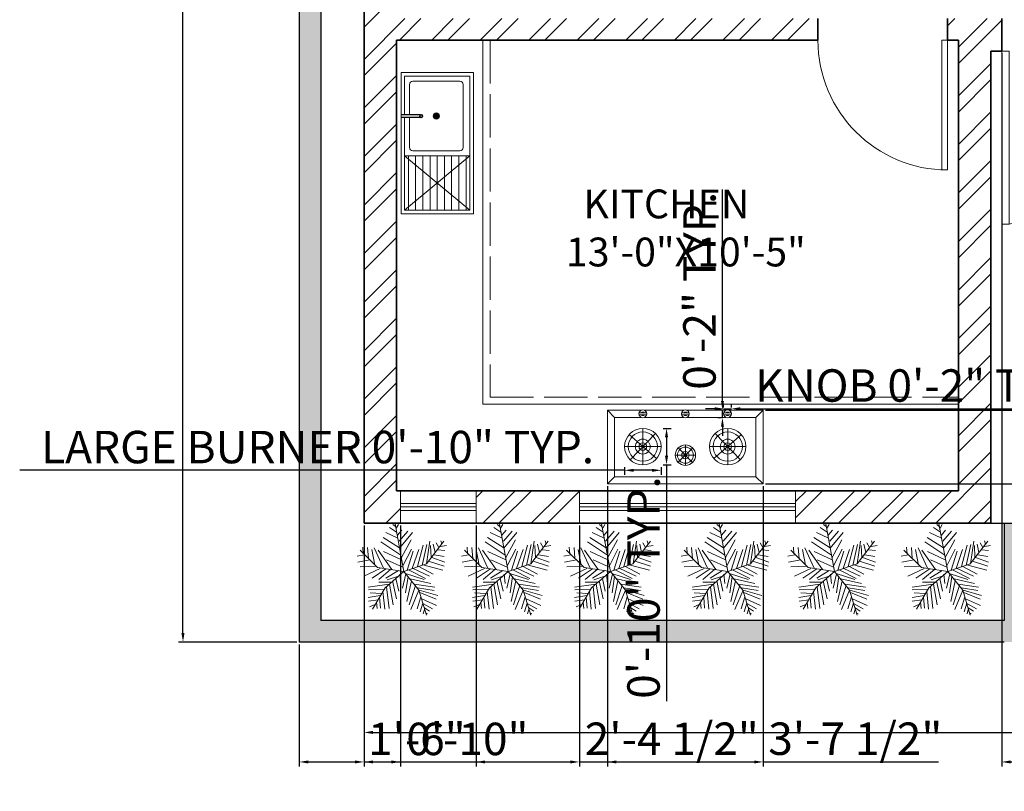
# Model space of a CAD drawing. Units: inches. Extents: x 418 to 1041, y 2094 to 2761.
# Tile 1 of 5: x 450 to 723, y 2094 to 2308. Entities that reach past the tile are written whole.
import ezdxf

# ---------------------------------------------------------------- set-up
doc = ezdxf.new("R2010")
doc.units = ezdxf.units.IN
doc.linetypes.add('ACAD_ISO02W100', pattern=[15, 12, -3])
for name, color, linetype, lineweight in [('A-ANNO-DIMS', 2, 'Continuous', 18), ('A-AREA-IDEN', 7, 'Continuous', 18), ('A-DOOR', 4, 'Continuous', 18), ('A-EQPM', 8, 'Continuous', 18), ('A-FLOR', 7, 'Continuous', 25), ('A-FLOR-CASE', 9, 'Continuous', 18), ('A-FLOR-CASE-HIDN', 9, 'ACAD_ISO02W100', 13), ('A-FLOR-FIXT', 9, 'Continuous', 18), ('A-GLAZ', 244, 'Continuous', 18), ('A-WALL', 7, 'Continuous', 35), ('A-WALL-PATT', 252, 'Continuous', 13), ('L-PLNT', 3, 'Continuous', 13), ('L-WALL', 7, 'Continuous', 25), ('L-WALL-PATT', 252, 'Continuous', 13)]:
    doc.layers.add(name, color=color, linetype=linetype, lineweight=lineweight)
doc.styles.get("Standard").update_dxf_attribs({"font": 'arial.ttf'})
doc.dimstyles.new('ISO-25', dxfattribs={"dimtxt": 9, "dimasz": 2.5, "dimexe": 1.25, "dimexo": 0.625, "dimtad": 1, "dimlunit": 3, "dimtxsty": 'Standard', "dimcen": 2.5, "dimadec": 0, "dimazin": 0, "dimtfac": 1, "dimtmove": 0, "dimatfit": 3, "dimfxl": 1, "dimarcsym": 0})

# ---------------------------------------------------------------- blocks, each defined once
blk = doc.blocks.new('*U3')
for p, q in [((0, 0), (0, 6)), ((40, 0), (40, 6))]:
    blk.add_line(p, q)
blk.add_lwpolyline([(0, 0), (0, -40), (1.75, -40), (1.75, 0)], close=True)
blk.add_arc((0, 0), 40, 270, 0)
blk = doc.blocks.new('*U4')
for p, q in [((-40, 0), (-40, 6)), ((0, 0), (0, 6))]:
    blk.add_line(p, q)
blk.add_lwpolyline([(0, 0), (0, -40), (-1.75, -40), (-1.75, 0)], close=True)
blk.add_arc((0, 0), 40, 180, 270)
blk = doc.blocks.new('*U14')
for p, q in [((-8.737, 47.138), (-17.069, 52.711)), ((-10.186, 53.64), (-13.084, 55.962)), ((0, 0), (-10.5, 57)), ((-9.099, 51.782), (-6.563, 55.962)), ((-7.65, 43.423), (-2.578, 49.46)), ((-5.839, 35.992), (4.667, 48.067)), ((-3.665, 19.273), (-27.574, 35.527)), ((-5.114, 28.097), (-24.676, 40.636)), ((-7.288, 39.707), (-21.778, 46.673)), ((-5.114, 27.632), (10.463, 46.673)), ((-2.941, 16.486), (8.652, 37.85)), ((27, 9), (48, 36)), ((27.127, 9.056), (31.112, 35.992)), ((44.153, 36.456), (45.239, 32.741)), ((-31.5, 4.5), (-52.5, 25.5)), ((-48.585, 21.131), (-49.309, 29.026)), ((-43.513, 28.561), (-42.427, 15.558)), ((-38.442, 26.239), (-34.819, 7.663)), ((-35.544, 28.097), (-24.314, 3.947)), ((-14.533, 2.09), (-30.834, 25.31)), ((-24.314, 23.917), (-2.941, 13.7)), ((-1.129, 6.734), (9.014, 26.704)), ((3.942, 1.625), (11.187, 24.381)), ((10.101, 3.483), (17.708, 26.239)), ((16.259, 5.805), (23.142, 31.348)), ((22.055, 7.198), (27.489, 32.277)), ((31.836, 30.883), (32.561, 16.486)), ((35.096, 32.741), (37.27, 22.524)), ((38.719, 34.134), (41.979, 28.561)), ((40.53, 25.775), (48.862, 24.846)), ((43.791, 29.954), (51.036, 30.883)), ((-47.498, 19.737), (-55.83, 18.344)), ((-40.615, 13.7), (-55.105, 10.913)), ((-20.691, 13.7), (-1.129, 4.876)), ((29.662, 12.307), (48.137, 6.269)), ((33.285, 16.486), (48.862, 10.913)), ((36.183, 19.737), (48.137, 17.88)), ((-33.37, 6.269), (-52.207, 5.34)), ((-28.299, 3.483), (-47.86, -5.805)), ((-21.416, 3.018), (-38.079, -8.128)), ((0, 0), (-31.5, 4.5)), ((-15.982, 2.09), (-30.11, -9.521)), ((0, 0), (-22.5, -19.5)), ((-6.563, 1.161), (-21.416, -8.128)), ((0, 0), (27, 9)), ((0, 0), (18, -22.5)), ((6.478, 1.625), (26.04, -8.592)), ((11.187, 3.483), (30.749, -5.805)), ((18.07, 5.805), (35.096, -3.483)), ((24.229, 7.663), (46.688, 1.625)), ((-6.563, -5.805), (-19.967, -9.985)), ((-13.446, -11.378), (-8.737, -32.741)), ((-9.461, -8.592), (-6.201, -23.453)), ((-4.752, -3.483), (-3.665, -14.629)), ((2.493, -3.019), (-1.491, -20.202)), ((1.769, -2.555), (24.229, -9.521)), ((5.029, -6.27), (2.131, -25.775)), ((9.014, -11.378), (3.58, -35.992)), ((7.565, -9.056), (32.198, -14.629)), ((-17.431, -15.094), (-42.789, -18.809)), ((-24.314, -21.596), (-42.427, -22.06)), ((-22.5, -19.5), (-37.5, -45)), ((-15.257, -12.772), (-30.11, -12.772)), ((-20.691, -18.345), (-17.793, -44.352)), ((-17.069, -15.094), (-12.721, -40.172)), ((14.085, -16.951), (6.478, -40.172)), ((18.07, -22.524), (8.289, -45.745)), ((12.274, -15.094), (36.907, -18.809)), ((16.259, -19.738), (36.183, -22.989)), ((18, -22.5), (27, -52.5)), ((18.433, -22.524), (40.53, -29.026)), ((-28.299, -29.026), (-42.789, -31.348)), ((-30.834, -34.135), (-42.427, -35.528)), ((-26.849, -26.24), (-40.253, -25.775)), ((-29.023, -30.884), (-27.936, -43.887)), ((-25.038, -23.918), (-22.865, -45.281)), ((20.244, -30.419), (15.897, -44.816)), ((19.157, -25.311), (38.719, -33.206)), ((21.331, -32.741), (39.081, -40.636)), ((-34.457, -39.708), (-40.978, -42.494)), ((-32.646, -36.921), (-31.921, -44.352)), ((22.78, -37.85), (19.519, -48.532)), ((22.78, -38.314), (34.372, -44.816)), ((24.591, -45.745), (23.142, -50.854)), ((24.591, -43.423), (30.749, -47.603)), ((26.764, -49.925), (28.213, -50.854))]:
    blk.add_line(p, q)
blk = doc.blocks.new('*D17')
at = {"layer": 'A-ANNO-DIMS', "color": 0, "lineweight": -2, "transparency": 16777216}
for p, q in [((545.56, 2167.4), (545.56, 2108.72)), ((971.56, 2167.4), (971.56, 2108.72)), ((548.06, 2109.97), (969.06, 2109.97))]:
    blk.add_line(p, q, dxfattribs=at)
at = {"layer": 'A-ANNO-DIMS', "color": 0, "transparency": 16777216}
for points in [[(548.06, 2110.39), (548.06, 2109.55), (545.56, 2109.97)], [(969.06, 2110.39), (969.06, 2109.55), (971.56, 2109.97)]]:
    blk.add_solid(points, dxfattribs=at)
at = {"layer": 'Defpoints', "color": 0, "transparency": 16777216}
for p in [(545.56, 2168.03), (971.56, 2168.03), (971.56, 2109.97)]:
    blk.add_point(p, dxfattribs=at)
at = {"layer": 'A-ANNO-DIMS', "color": 0, "transparency": 16777216, "insert": (758.56, 2115.19), "char_height": 9, "attachment_point": 5}
blk.add_mtext('35\'-6"', dxfattribs=at)
blk = doc.blocks.new('WIN-60IN')
for p, q in [((0, 5.5), (60, 5.5)), ((0, 4.5), (60, 4.5)), ((0, 3.5), (60, 3.5))]:
    blk.add_line(p, q)
blk.add_lwpolyline([(0, 9), (60, 9), (60, 0), (0, 0)], close=True)
blk = doc.blocks.new('WIN-21IN')
for p, q in [((0, 5.5), (21, 5.5)), ((0, 4.5), (21, 4.5)), ((0, 3.5), (21, 3.5))]:
    blk.add_line(p, q)
blk.add_lwpolyline([(0, 9), (21, 9), (21, 0), (0, 0)], close=True)
blk = doc.blocks.new('COOKTOP-BURNER-LARGE')
for p, q in [((1.24, 8.38), (8.89, 1.74)), ((8.59, 8.7), (1.54, 1.43)), ((5.06, 0), (5.06, 10.12)), ((10.12, 5.06), (0, 5.06))]:
    blk.add_line(p, q)
for radius in [5.06, 4.06, 2.06, 1.06]:
    blk.add_circle((5.06, 5.06), radius)
blk = doc.blocks.new('COOKTOP-CONTROL')
for p, q in [((2.12, 1.38), (0.04, 1.38)), ((2.12, 0.78), (0.04, 0.78))]:
    blk.add_line(p, q)
blk.add_circle((1.08, 1.08), 1.08)
for start, end in [(38.584, 141.416), (218.584, 321.416)]:
    blk.add_arc((1.08, 1.08), 0.481, start, end)
blk = doc.blocks.new('*D29')
at = {"layer": 'A-ANNO-DIMS', "color": 0, "lineweight": -2, "transparency": 16777216}
for p, q in [((645.38, 2200.08), (645.38, 2201.03)), ((647.54, 2200.08), (647.54, 2201.03)), ((642.88, 2199.78), (640.38, 2199.78)), ((645.38, 2199.78), (647.54, 2199.78)), ((650.04, 2199.78), (747.37, 2199.78))]:
    blk.add_line(p, q, dxfattribs=at)
at = {"layer": 'A-ANNO-DIMS', "color": 0, "transparency": 16777216}
for points in [[(642.88, 2200.2), (642.88, 2199.36), (645.38, 2199.78)], [(650.04, 2200.2), (650.04, 2199.36), (647.54, 2199.78)]]:
    blk.add_solid(points, dxfattribs=at)
at = {"layer": 'Defpoints', "color": 0, "transparency": 16777216}
for p in [(645.38, 2199.46), (647.54, 2199.78), (647.54, 2199.46)]:
    blk.add_point(p, dxfattribs=at)
at = {"layer": 'A-ANNO-DIMS', "color": 0, "transparency": 16777216, "insert": (699.96, 2205.06), "char_height": 9, "attachment_point": 5}
blk.add_mtext('KNOB 0\'-2" TYP.', dxfattribs=at)
blk = doc.blocks.new('*D30')
at = {"layer": 'A-ANNO-DIMS', "color": 0, "lineweight": -2, "transparency": 16777216}
for p, q in [((645.05, 2201.96), (645.05, 2260.57)), ((644.75, 2199.46), (643.8, 2199.46)), ((645.05, 2197.29), (645.05, 2199.46)), ((644.75, 2197.29), (643.8, 2197.29)), ((645.05, 2194.79), (645.05, 2192.29))]:
    blk.add_line(p, q, dxfattribs=at)
at = {"layer": 'A-ANNO-DIMS', "color": 0, "transparency": 16777216}
for points in [[(644.64, 2201.96), (645.47, 2201.96), (645.05, 2199.46)], [(644.64, 2194.79), (645.47, 2194.79), (645.05, 2197.29)]]:
    blk.add_solid(points, dxfattribs=at)
at = {"layer": 'Defpoints', "color": 0, "transparency": 16777216}
for p in [(645.05, 2199.46), (645.38, 2199.46), (645.38, 2197.29)]:
    blk.add_point(p, dxfattribs=at)
at = {"layer": 'A-ANNO-DIMS', "color": 0, "transparency": 16777216, "insert": (639.83, 2232.51), "char_height": 9, "attachment_point": 5, "rotation": 90}
blk.add_mtext('0\'-2" TYP.', dxfattribs=at)
blk = doc.blocks.new('*D31')
at = {"layer": 'A-ANNO-DIMS', "color": 0, "lineweight": -2, "transparency": 16777216}
for p, q in [((617.89, 2182.7), (449.98, 2182.7)), ((617.89, 2183.59), (617.89, 2181.45)), ((625.51, 2182.7), (620.39, 2182.7)), ((628.01, 2183.59), (628.01, 2181.45))]:
    blk.add_line(p, q, dxfattribs=at)
at = {"layer": 'A-ANNO-DIMS', "color": 0, "transparency": 16777216}
for points in [[(620.39, 2183.11), (620.39, 2182.28), (617.89, 2182.7)], [(625.51, 2183.11), (625.51, 2182.28), (628.01, 2182.7)]]:
    blk.add_solid(points, dxfattribs=at)
at = {"layer": 'Defpoints', "color": 0, "transparency": 16777216}
for p in [(617.89, 2184.22), (628.01, 2184.22), (617.89, 2182.7)]:
    blk.add_point(p, dxfattribs=at)
at = {"layer": 'A-ANNO-DIMS', "color": 0, "transparency": 16777216, "insert": (532.68, 2187.98), "char_height": 9, "attachment_point": 5}
blk.add_mtext('LARGE BURNER 0\'-10" TYP.', dxfattribs=at)
blk = doc.blocks.new('*D32')
at = {"layer": 'A-ANNO-DIMS', "color": 0, "lineweight": -2, "transparency": 16777216}
for p, q in [((628.64, 2194.34), (630.78, 2194.34)), ((629.53, 2191.84), (629.53, 2186.72)), ((628.64, 2184.22), (630.78, 2184.22)), ((629.53, 2184.22), (629.53, 2118.61))]:
    blk.add_line(p, q, dxfattribs=at)
at = {"layer": 'A-ANNO-DIMS', "color": 0, "transparency": 16777216}
for points in [[(629.11, 2191.84), (629.95, 2191.84), (629.53, 2194.34)], [(629.11, 2186.72), (629.95, 2186.72), (629.53, 2184.22)]]:
    blk.add_solid(points, dxfattribs=at)
at = {"layer": 'Defpoints', "color": 0, "transparency": 16777216}
for p in [(628.01, 2194.34), (628.01, 2184.22), (629.53, 2184.22)]:
    blk.add_point(p, dxfattribs=at)
at = {"layer": 'A-ANNO-DIMS', "color": 0, "transparency": 16777216, "insert": (624.31, 2150.17), "char_height": 9, "attachment_point": 5, "rotation": 90}
blk.add_mtext('0\'-10" TYP.', dxfattribs=at)
blk = doc.blocks.new('*D51')
at = {"layer": 'A-ANNO-DIMS', "color": 0, "lineweight": -2, "transparency": 16777216}
for p, q in [((545.56, 2167.4), (545.56, 2100.53)), ((555.67, 2167.4), (555.67, 2100.53)), ((548.06, 2101.78), (553.17, 2101.78)), ((555.67, 2101.78), (590.33, 2101.78))]:
    blk.add_line(p, q, dxfattribs=at)
at = {"layer": 'A-ANNO-DIMS', "color": 0, "transparency": 16777216}
for points in [[(548.06, 2102.19), (548.06, 2101.36), (545.56, 2101.78)], [(553.17, 2102.19), (553.17, 2101.36), (555.67, 2101.78)]]:
    blk.add_solid(points, dxfattribs=at)
at = {"layer": 'Defpoints', "color": 0, "transparency": 16777216}
for p in [(545.56, 2168.03), (555.67, 2168.03), (555.67, 2101.78)]:
    blk.add_point(p, dxfattribs=at)
at = {"layer": 'A-ANNO-DIMS', "color": 0, "transparency": 16777216, "insert": (574.25, 2107), "char_height": 9, "attachment_point": 5}
blk.add_mtext('0\'-10"', dxfattribs=at)
blk = doc.blocks.new('*D52')
at = {"layer": 'A-ANNO-DIMS', "color": 0, "lineweight": -2, "transparency": 16777216}
for p, q in [((576.67, 2167.4), (576.67, 2100.53)), ((605.34, 2167.4), (605.34, 2100.53)), ((579.17, 2101.78), (602.84, 2101.78)), ((605.34, 2101.78), (654.14, 2101.78))]:
    blk.add_line(p, q, dxfattribs=at)
at = {"layer": 'A-ANNO-DIMS', "color": 0, "transparency": 16777216}
for points in [[(579.17, 2102.19), (579.17, 2101.36), (576.67, 2101.78)], [(602.84, 2102.19), (602.84, 2101.36), (605.34, 2101.78)]]:
    blk.add_solid(points, dxfattribs=at)
at = {"layer": 'Defpoints', "color": 0, "transparency": 16777216}
for p in [(576.67, 2168.03), (605.34, 2168.03), (605.34, 2101.78)]:
    blk.add_point(p, dxfattribs=at)
at = {"layer": 'A-ANNO-DIMS', "color": 0, "transparency": 16777216, "insert": (630.99, 2107.05), "char_height": 9, "attachment_point": 5}
blk.add_mtext('2\'-4 1/2"', dxfattribs=at)
blk = doc.blocks.new('*D57')
at = {"layer": 'A-ANNO-DIMS', "color": 0, "lineweight": -2, "transparency": 16777216}
for p, q in [((722.56, 2298.4), (722.56, 2100.53)), ((770.56, 2298.4), (770.56, 2100.53)), ((725.06, 2101.78), (768.06, 2101.78))]:
    blk.add_line(p, q, dxfattribs=at)
at = {"layer": 'A-ANNO-DIMS', "color": 0, "transparency": 16777216}
for points in [[(725.06, 2102.19), (725.06, 2101.36), (722.56, 2101.78)], [(768.06, 2102.19), (768.06, 2101.36), (770.56, 2101.78)]]:
    blk.add_solid(points, dxfattribs=at)
at = {"layer": 'Defpoints', "color": 0, "transparency": 16777216}
for p in [(722.56, 2299.03), (770.56, 2299.03), (770.56, 2101.78)]:
    blk.add_point(p, dxfattribs=at)
at = {"layer": 'A-ANNO-DIMS', "color": 0, "transparency": 16777216, "insert": (746.56, 2107), "char_height": 9, "attachment_point": 5}
blk.add_mtext('4\'-0"', dxfattribs=at)
blk = doc.blocks.new('*D61')
at = {"layer": 'A-ANNO-DIMS', "color": 0, "lineweight": -2, "transparency": 16777216}
for p, q in [((526.93, 2684.03), (494.06, 2684.03)), ((495.31, 2137.53), (495.31, 2681.53)), ((526.93, 2135.03), (494.06, 2135.03))]:
    blk.add_line(p, q, dxfattribs=at)
at = {"layer": 'A-ANNO-DIMS', "color": 0, "transparency": 16777216}
for points in [[(494.89, 2681.53), (495.72, 2681.53), (495.31, 2684.03)], [(494.89, 2137.53), (495.72, 2137.53), (495.31, 2135.03)]]:
    blk.add_solid(points, dxfattribs=at)
at = {"layer": 'Defpoints', "color": 0, "transparency": 16777216}
for p in [(495.31, 2684.03), (527.56, 2684.03), (527.56, 2135.03)]:
    blk.add_point(p, dxfattribs=at)
at = {"layer": 'A-ANNO-DIMS', "color": 0, "transparency": 16777216, "insert": (490.09, 2409.53), "char_height": 9, "attachment_point": 5, "rotation": 90}
blk.add_mtext('45\'-9"', dxfattribs=at)
blk = doc.blocks.new('*D66')
at = {"layer": 'A-ANNO-DIMS', "color": 0, "lineweight": -2, "transparency": 16777216}
for p, q in [((545.56, 2167.4), (545.56, 2100.53)), ((527.56, 2134.4), (527.56, 2100.53)), ((530.06, 2101.78), (543.06, 2101.78)), ((545.56, 2101.78), (572.38, 2101.78))]:
    blk.add_line(p, q, dxfattribs=at)
at = {"layer": 'A-ANNO-DIMS', "color": 0, "transparency": 16777216}
for points in [[(530.06, 2102.19), (530.06, 2101.36), (527.56, 2101.78)], [(543.06, 2102.19), (543.06, 2101.36), (545.56, 2101.78)]]:
    blk.add_solid(points, dxfattribs=at)
at = {"layer": 'Defpoints', "color": 0, "transparency": 16777216}
for p in [(545.56, 2168.03), (527.56, 2135.03), (545.56, 2101.78)]:
    blk.add_point(p, dxfattribs=at)
at = {"layer": 'A-ANNO-DIMS', "color": 0, "transparency": 16777216, "insert": (560.22, 2107), "char_height": 9, "attachment_point": 5}
blk.add_mtext('1\'-6"', dxfattribs=at)
blk = doc.blocks.new('*D68')
at = {"layer": 'A-ANNO-DIMS', "color": 0, "lineweight": -2, "transparency": 16777216}
for p, q in [((613.11, 2178.28), (613.11, 2100.53)), ((656.36, 2178.28), (656.36, 2100.53)), ((615.61, 2101.78), (653.86, 2101.78)), ((656.36, 2101.78), (705, 2101.78))]:
    blk.add_line(p, q, dxfattribs=at)
at = {"layer": 'A-ANNO-DIMS', "color": 0, "transparency": 16777216}
for points in [[(615.61, 2102.19), (615.61, 2101.36), (613.11, 2101.78)], [(653.86, 2102.19), (653.86, 2101.36), (656.36, 2101.78)]]:
    blk.add_solid(points, dxfattribs=at)
at = {"layer": 'Defpoints', "color": 0, "transparency": 16777216}
for p in [(613.11, 2178.9), (656.36, 2178.9), (656.36, 2101.78)]:
    blk.add_point(p, dxfattribs=at)
at = {"layer": 'A-ANNO-DIMS', "color": 0, "transparency": 16777216, "insert": (681.93, 2107.06), "char_height": 9, "attachment_point": 5}
blk.add_mtext('3\'-7 1/2"', dxfattribs=at)
blk = doc.blocks.new('*D69')
at = {"layer": 'A-ANNO-DIMS', "color": 0, "lineweight": -2, "transparency": 16777216}
for p, q in [((1022.01, 2199.37), (1022.01, 2247.17)), ((656.98, 2199.37), (1023.26, 2199.37)), ((1022.01, 2181.4), (1022.01, 2196.87)), ((656.98, 2178.9), (1023.26, 2178.9))]:
    blk.add_line(p, q, dxfattribs=at)
at = {"layer": 'A-ANNO-DIMS', "color": 0, "transparency": 16777216}
for points in [[(1021.6, 2196.87), (1022.43, 2196.87), (1022.01, 2199.37)], [(1021.6, 2181.4), (1022.43, 2181.4), (1022.01, 2178.9)]]:
    blk.add_solid(points, dxfattribs=at)
at = {"layer": 'Defpoints', "color": 0, "transparency": 16777216}
for p in [(656.36, 2199.37), (1022.01, 2199.37), (656.36, 2178.9)]:
    blk.add_point(p, dxfattribs=at)
at = {"layer": 'A-ANNO-DIMS', "color": 0, "transparency": 16777216, "insert": (1016.74, 2224.52), "char_height": 9, "attachment_point": 5, "rotation": 90}
blk.add_mtext('1\'-8 1/2"', dxfattribs=at)

msp = doc.modelspace()

# ---------------------------------------------------------------- hatches: boundary and pattern name
at = {"layer": 'A-WALL-PATT'}
h = msp.add_hatch(dxfattribs=at)
h.set_pattern_fill('ANSI32', color=256)
h.paths.add_polyline_path([(671.558, 2308.025), (554.558, 2308.025), (554.558, 2366.352), (545.558, 2366.352), (545.558, 2168.025), (555.667, 2168.025), (555.667, 2177.025), (554.558, 2177.025), (554.558, 2302.025), (671.558, 2302.025)])
h.paths.add_polyline_path([(719.558, 2299.025), (722.558, 2299.025), (722.558, 2306.225), (722.558, 2308.025), (707.558, 2308.025), (707.558, 2302.025), (710.558, 2302.025), (710.558, 2177.025), (665.344, 2177.025), (665.344, 2168.025), (719.558, 2168.025)])
h.paths.add_polyline_path([(605.344, 2177.025), (576.667, 2177.025), (576.667, 2168.025), (605.344, 2168.025)], flags=17)
h.paths.add_polyline_path([(795.654, 2308.025), (770.558, 2308.025), (770.558, 2299.025), (795.654, 2299.025)])
h.paths.add_polyline_path([(971.558, 2333.525), (962.558, 2333.525), (962.558, 2308.025), (890.558, 2308.025), (890.558, 2311.025), (886.058, 2311.025), (884.558, 2311.025), (884.558, 2308.025), (855.654, 2308.025), (855.654, 2299.025), (962.558, 2299.025), (962.558, 2269.763), (971.558, 2269.763)])
h.paths.add_polyline_path([(971.558, 2209.763), (962.558, 2209.763), (962.558, 2168.025), (971.558, 2168.025)])
h.paths.add_polyline_path([(971.558, 2422.525), (962.558, 2422.525), (962.558, 2386.025), (845.558, 2386.025), (845.558, 2380.025), (884.558, 2380.025), (884.558, 2341.025), (890.558, 2341.025), (890.558, 2380.025), (962.558, 2380.025), (962.558, 2354.525), (971.558, 2354.525)])
h.paths.add_polyline_path([(716.558, 2471.025), (651.558, 2471.025), (651.558, 2474.025), (647.058, 2474.025), (645.558, 2474.025), (645.558, 2471.025), (554.558, 2471.025), (554.558, 2484.525), (545.558, 2484.525), (545.558, 2426.352), (554.558, 2426.352), (554.558, 2465.025), (716.558, 2465.025)])
h.paths.add_polyline_path([(554.558, 2561.611), (545.558, 2561.611), (545.558, 2505.525), (554.558, 2505.525), (554.558, 2519.025), (645.558, 2519.025), (645.558, 2504.025), (651.558, 2504.025), (651.558, 2519.025), (716.558, 2519.025), (716.558, 2528.025), (710.558, 2528.025), (710.558, 2525.025), (554.558, 2525.025)])
h.paths.add_polyline_path([(971.558, 2561.025), (962.558, 2561.025), (962.558, 2525.025), (806.558, 2525.025), (806.558, 2528.025), (800.558, 2528.025), (800.558, 2380.025), (809.558, 2380.025), (809.558, 2386.025), (806.558, 2386.025), (806.558, 2519.025), (962.558, 2519.025), (962.558, 2482.525), (971.558, 2482.525)])
h.paths.add_polyline_path([(854.558, 2666.025), (769.058, 2666.025), (769.058, 2657.025), (800.558, 2657.025), (800.558, 2589.025), (797.558, 2589.025), (797.558, 2583.025), (800.558, 2583.025), (800.558, 2564.025), (806.558, 2564.025), (806.558, 2657.025), (854.558, 2657.025)])
h.paths.add_polyline_path([(971.558, 2666.025), (914.558, 2666.025), (914.558, 2657.025), (962.558, 2657.025), (962.558, 2621.025), (971.558, 2621.025)])
h.paths.add_polyline_path([(748.058, 2666.025), (662.558, 2666.025), (662.558, 2657.025), (710.558, 2657.025), (710.558, 2564.025), (716.558, 2564.025), (716.558, 2583.025), (767.558, 2583.025), (767.558, 2589.025), (716.558, 2589.025), (716.558, 2657.025), (748.058, 2657.025)])
h.paths.add_polyline_path([(602.558, 2666.025), (545.558, 2666.025), (545.558, 2621.611), (554.558, 2621.611), (554.558, 2657.025), (602.558, 2657.025)])
at = {"layer": 'L-WALL-PATT'}
h = msp.add_hatch(color=256, dxfattribs=at)
h.dxf.hatch_style = 1
h.paths.add_polyline_path([(533.558, 2678.025), (983.558, 2678.025), (983.558, 2141.025), (902.558, 2141.025), (902.558, 2168.025), (893.558, 2168.025), (893.558, 2135.025), (926.558, 2135.025), (989.558, 2135.025), (989.558, 2684.025), (527.558, 2684.025), (527.558, 2135.025), (723.29, 2135.025), (732.29, 2135.025), (732.29, 2168.025), (723.29, 2168.025), (723.29, 2141.025), (533.558, 2141.025)])

# ---------------------------------------------------------------- linework, layer by layer
at = {"layer": 'A-EQPM'}
for p, q in [((613.107, 2199.375), (615.107, 2197.375)), ((654.359, 2197.375), (656.359, 2199.375)), ((634.765, 2189.722), (634.765, 2184.073)), ((631.94, 2186.898), (637.59, 2186.898)), ((632.758, 2184.91), (636.772, 2188.885)), ((636.766, 2184.904), (632.764, 2188.891)), ((613.107, 2178.9), (615.107, 2180.9)), ((654.359, 2180.9), (656.359, 2178.9))]:
    msp.add_line(p, q, dxfattribs=at)
for points in [[(646.868, 2199.375), (656.359, 2199.375), (656.359, 2178.9), (613.107, 2178.9), (613.107, 2199.375), (622.537, 2199.375)], [(623.359, 2199.375), (634.363, 2199.375)], [(635.167, 2199.375), (646.047, 2199.375)], [(646.868, 2197.375), (654.359, 2197.375), (654.359, 2180.9), (615.107, 2180.9), (615.107, 2197.375), (622.537, 2197.375)], [(623.359, 2197.375), (634.346, 2197.375)], [(635.184, 2197.375), (646.047, 2197.375)]]:
    msp.add_lwpolyline(points, dxfattribs=at)
for radius in [2.825, 2.225, 1.025, 0.425]:
    msp.add_circle((634.765, 2186.898), radius, dxfattribs=at)
at = {"layer": 'A-FLOR'}
msp.add_line((719.558, 2168.025), (962.558, 2168.025), dxfattribs=at)
at = {"layer": 'A-FLOR-CASE'}
for p, q in [((578.558, 2302.025), (578.558, 2201.025)), ((578.558, 2201.025), (710.558, 2201.025))]:
    msp.add_line(p, q, dxfattribs=at)
at = {"layer": 'A-FLOR-CASE-HIDN'}
for p, q in [((580.558, 2302.025), (580.558, 2203.025)), ((580.558, 2203.025), (710.558, 2203.025))]:
    msp.add_line(p, q, dxfattribs=at)
at = {"layer": 'A-FLOR-FIXT'}
for p, q in [((555.827, 2281.393), (561.214, 2281.393)), ((555.827, 2281.293), (561.098, 2281.293)), ((555.827, 2280.693), (561.098, 2280.693)), ((555.827, 2280.593), (561.214, 2280.593)), ((564.732, 2280.993), (566.502, 2280.993)), ((566.433, 2280.652), (564.801, 2281.335)), ((564.811, 2280.627), (566.423, 2281.359)), ((566.261, 2280.386), (564.973, 2281.6)), ((564.986, 2280.373), (566.248, 2281.614)), ((565.957, 2280.176), (565.277, 2281.81)), ((565.325, 2280.158), (565.909, 2281.828)), ((565.617, 2281.878), (565.617, 2280.108)), ((556.827, 2269.953), (574.934, 2269.953)), ((556.827, 2269.953), (574.934, 2254.833)), ((556.827, 2254.833), (574.934, 2269.953)), ((557.881, 2269.953), (557.881, 2254.833)), ((559.881, 2269.953), (559.881, 2254.833)), ((561.881, 2269.953), (561.881, 2254.833)), ((563.881, 2269.953), (563.881, 2254.833)), ((563.881, 2269.953), (563.881, 2254.833)), ((565.881, 2269.953), (565.881, 2254.833)), ((567.881, 2269.953), (567.881, 2254.833)), ((569.881, 2269.953), (569.881, 2254.833)), ((571.881, 2269.953), (571.881, 2254.833)), ((573.881, 2269.953), (573.881, 2254.833))]:
    msp.add_line(p, q, dxfattribs=at)
msp.add_lwpolyline([(555.827, 2293.051), (575.934, 2293.051), (575.934, 2253.833), (555.827, 2253.833)], close=True, dxfattribs=at)
msp.add_lwpolyline([(556.827, 2281.393), (556.827, 2292.051), (574.934, 2292.051), (574.934, 2254.833), (556.827, 2254.833), (556.827, 2280.593)], dxfattribs=at)
msp.add_lwpolyline([(558.186, 2281.393), (558.186, 2289.756, -0.4142136), (559.086, 2290.656), (572.148, 2290.656, -0.4142136), (573.048, 2289.756), (573.048, 2272.231, -0.4142136), (572.148, 2271.331), (559.086, 2271.331, -0.4142136), (558.186, 2272.231), (558.186, 2280.593)], format="xyb", dxfattribs=at)
for centre, radius in [((561.459, 2280.993), 0.469), ((561.459, 2280.993), 0.269), ((565.617, 2280.993), 0.885), ((565.617, 2280.993), 0.685)]:
    msp.add_circle(centre, radius, dxfattribs=at)
at = {"layer": 'A-WALL'}
for p, q in [((545.558, 2666.025), (545.558, 2168.025)), ((671.558, 2302.025), (671.558, 2308.025)), ((707.558, 2302.025), (707.558, 2308.025)), ((722.558, 2299.025), (722.558, 2308.025)), ((554.558, 2302.025), (671.558, 2302.025)), ((554.558, 2302.025), (554.558, 2177.025)), ((707.558, 2302.025), (710.558, 2302.025)), ((710.558, 2302.025), (710.558, 2177.025)), ((719.558, 2299.025), (719.558, 2168.025)), ((719.558, 2299.025), (722.558, 2299.025)), ((554.558, 2177.025), (710.558, 2177.025)), ((545.558, 2168.025), (719.558, 2168.025))]:
    msp.add_line(p, q, dxfattribs=at)
at = {"layer": 'L-WALL'}
for p, q in [((527.558, 2684.025), (527.558, 2135.025)), ((533.558, 2678.025), (533.558, 2141.025)), ((723.29, 2168.025), (723.29, 2141.025)), ((723.29, 2141.025), (533.558, 2141.025)), ((723.29, 2135.025), (527.558, 2135.025))]:
    msp.add_line(p, q, dxfattribs=at)

# ---------------------------------------------------------------- block references
at = {"layer": 'A-DOOR'}
for name, p, xscale, yscale, zscale in [('*U4', (707.558, 2302.025), 0.9, 0.9, 0.9), ('*U3', (722.558, 2299.025), 1.199999999999997, 1.199999999999997, 1.199999999999997)]:
    msp.add_blockref(name, p, dxfattribs=dict(at, xscale=xscale, yscale=yscale, zscale=zscale))
at = {"layer": 'A-EQPM', "rotation": 180}
for name, p in [('COOKTOP-CONTROL', (624.029, 2199.456)), ('COOKTOP-BURNER-LARGE', (628.01, 2194.34))]:
    msp.add_blockref(name, p, dxfattribs=at)
at = {"layer": 'A-EQPM'}
for p in [(633.684, 2197.29), (645.377, 2197.294)]:
    msp.add_blockref('COOKTOP-CONTROL', p, dxfattribs=at)
at = {"layer": 'A-EQPM', "extrusion": (0, 0, -1), "zscale": -1, "rotation": 180}
msp.add_blockref('COOKTOP-BURNER-LARGE', (-641.455, 2194.34), dxfattribs=at)
at = {"layer": 'A-GLAZ'}
for name, p in [('WIN-21IN', (555.667, 2168.025)), ('WIN-60IN', (605.344, 2168.025))]:
    msp.add_blockref(name, p, dxfattribs=at)
at = {"layer": 'L-PLNT', "xscale": 0.2319011365265418, "yscale": 0.2319011365265418, "zscale": 0.2319011365265418}
for p in [(556.624, 2154.646), (585.588, 2154.646), (613.949, 2154.646), (646.57, 2154.646), (676.172, 2154.646), (707.592, 2154.646)]:
    msp.add_blockref('*U14', p, dxfattribs=at)

# ---------------------------------------------------------------- texts
at = {"layer": 'A-AREA-IDEN', "insert": (601.597, 2260.605), "char_height": 8, "attachment_point": 1}
msp.add_mtext_dynamic_manual_height_columns('  KITCHEN\\P13\'-0"X10\'-5"', width=63.10181, gutter_width=12.5, heights=[0], dxfattribs=at)

# ---------------------------------------------------------------- dimensions: what is measured, and where the dimension line sits
at = {"layer": 'A-ANNO-DIMS'}
for base, p1, p2, picture, middle in [((495.308, 2684.025), (527.558, 2135.025), (527.558, 2684.025), '*D61', (490.088, 2409.525)), ((1022.015, 2199.375), (656.359, 2178.9), (656.359, 2199.375), '*D69', (1016.736, 2224.524))]:
    dim = msp.add_linear_dim(base=base, p1=p1, p2=p2, angle=90, dimstyle='ISO-25', override={"dimdec": 1, "dimlfac": 1, "dimrnd": 0, "dimzin": 1, "dimdsep": 46, "dimlunit": 4, "dimfrac": 2}, dxfattribs=at)
    dim.commit()
    dim.dimension.update_dxf_attribs({"geometry": picture, "text_midpoint": middle})
for base, p1, p2, override, picture, middle in [((770.558, 2101.775), (722.558, 2299.025), (770.558, 2299.025), {"dimdec": 1, "dimlfac": 1, "dimrnd": 0, "dimzin": 1, "dimdsep": 46, "dimlunit": 4, "dimfrac": 2}, '*D57', (746.558, 2106.996)), ((656.359, 2101.775), (613.107, 2178.9), (656.359, 2178.9), {"dimdec": 1, "dimlfac": 1, "dimrnd": 0, "dimzin": 1, "dimdsep": 46, "dimlunit": 4, "dimfrac": 2}, '*D68', (681.928, 2107.057)), ((545.558, 2101.775), (527.558, 2135.025), (545.558, 2168.025), {"dimdec": 1, "dimlfac": 1, "dimrnd": 0, "dimzin": 1, "dimdsep": 46, "dimlunit": 4, "dimfrac": 2}, '*D66', (560.221, 2106.996)), ((971.558, 2109.971), (545.558, 2168.025), (971.558, 2168.025), {"dimclrd": 0, "dimclre": 0, "dimclrt": 0}, '*D17', (758.558, 2115.194)), ((555.667, 2101.775), (545.558, 2168.025), (555.667, 2168.025), {"dimdec": 1, "dimlfac": 1, "dimrnd": 0, "dimzin": 1, "dimdsep": 46, "dimlunit": 4, "dimfrac": 2}, '*D51', (574.25, 2106.996)), ((605.344, 2101.775), (576.667, 2168.025), (605.344, 2168.025), {"dimdec": 1, "dimlfac": 1, "dimrnd": 0, "dimzin": 1, "dimdsep": 46, "dimlunit": 4, "dimfrac": 2}, '*D52', (630.993, 2107.054))]:
    dim = msp.add_linear_dim(base=base, p1=p1, p2=p2, dimstyle='ISO-25', override=override, dxfattribs=at)
    dim.commit()
    dim.dimension.update_dxf_attribs({"geometry": picture, "text_midpoint": middle})
for base, p1, p2, angle, text, picture, middle in [((645.052, 2199.456), (645.377, 2197.294), (645.377, 2199.456), 90, '<> TYP.', '*D30', (639.832, 2232.511)), ((617.886, 2182.697), (628.01, 2184.216), (617.886, 2184.216), 180, 'LARGE BURNER <> TYP.', '*D31', (532.683, 2187.976)), ((629.529, 2184.216), (628.01, 2194.34), (628.01, 2184.216), 270, '<> TYP.', '*D32', (624.309, 2150.165))]:
    dim = msp.add_linear_dim(base=base, p1=p1, p2=p2, angle=angle, text=text, dimstyle='ISO-25', override={"dimdec": 1, "dimlfac": 1, "dimrnd": 0, "dimzin": 1, "dimdsep": 46, "dimlunit": 4, "dimfrac": 2}, dxfattribs=at)
    dim.commit()
    dim.dimension.update_dxf_attribs({"geometry": picture, "text_midpoint": middle})
dim = msp.add_linear_dim(base=(647.539, 2199.78), p1=(645.377, 2199.456), p2=(647.539, 2199.456), text='KNOB <> TYP.', dimstyle='ISO-25', override={"dimdec": 1, "dimlfac": 1, "dimrnd": 0, "dimzin": 1, "dimdsep": 46, "dimlunit": 4, "dimfrac": 2}, dxfattribs=at)
dim.commit()
dim.dimension.update_dxf_attribs({"geometry": '*D29', "text_midpoint": (699.956, 2205.062)})

doc.saveas('drawing.dxf')
